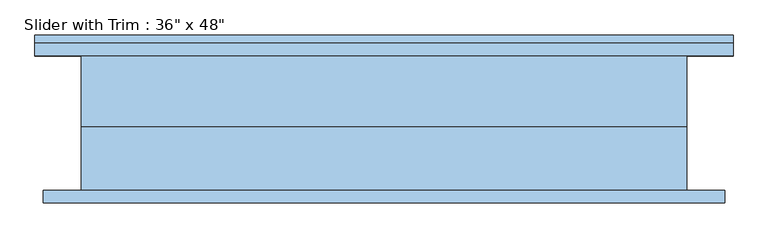
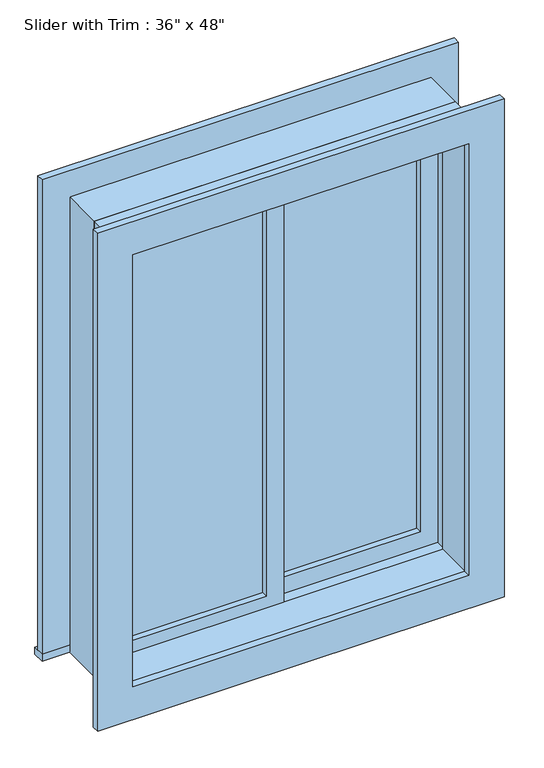
"""IFC4 building model written with IfcOpenShell, lengths in millimetres: window geometry."""

from ifc_helpers import new_model, si_unit, frame, origin, place, context, project, spatial, polyline, outline, extrude, source, transform, mapped, element, save


def window_54100e87(model_context):
    return source(origin(), model_context, "Body", "SweptSolid", [
        extrude(outline(polyline([(-393.7, 22.225), (-22.225, 22.225), (-22.225, 9.525), (-393.7, 9.525), (-393.7, 22.225)])), frame((0.0, 0.0, 977.9), z_axis=(0.0, 0.0, 1.0), x_axis=(1.0, 0.0, 0.0)), (0.0, 0.0, 1.0), 1092.2),
        extrude(outline(polyline([(2114.55, -438.15), (933.45, -438.15), (933.45, 22.225), (2114.55, 22.225), (2114.55, -438.15)]), holes=[polyline([(2070.1, -393.7), (2070.1, -22.225), (977.9, -22.225), (977.9, -393.7), (2070.1, -393.7)])]), frame((0.0, -6.35, 0.0), z_axis=(0.0, 1.0, 0.0), x_axis=(0.0, 0.0, 1.0)), (0.0, 0.0, 1.0), 44.45),
        extrude(outline(polyline([(-527.05, 133.35), (527.05, 133.35), (527.05, 101.6), (-527.05, 101.6), (-527.05, 133.35)])), frame((0.0, 0.0, 914.4), z_axis=(0.0, 0.0, 1.0), x_axis=(1.0, 0.0, 0.0)), (0.0, 0.0, 1.0), 19.05),
        extrude(outline(polyline([(2114.55, -438.15), (2114.55, 438.15), (933.45, 438.15), (933.45, 527.05), (2203.45, 527.05), (2203.45, -527.05), (933.45, -527.05), (933.45, -438.15), (2114.55, -438.15)])), frame((0.0, 101.6, 0.0), z_axis=(0.0, 1.0, 0.0), x_axis=(0.0, 0.0, 1.0)), (0.0, 0.0, 1.0), 19.05),
        extrude(outline(polyline([(2190.75, 514.35), (2190.75, -514.35), (857.25, -514.35), (857.25, 514.35), (2190.75, 514.35)]), holes=[polyline([(2101.85, 425.45), (946.15, 425.45), (946.15, -425.45), (2101.85, -425.45), (2101.85, 425.45)])]), frame((0.0, -120.65, 0.0), z_axis=(0.0, 1.0, 0.0), x_axis=(0.0, 0.0, 1.0)), (0.0, 0.0, 1.0), 19.05),
        extrude(outline(polyline([(393.7, 53.975), (22.225, 53.975), (22.225, 66.675), (393.7, 66.675), (393.7, 53.975)])), frame((0.0, 0.0, 977.9), z_axis=(0.0, 0.0, 1.0), x_axis=(1.0, 0.0, 0.0)), (0.0, 0.0, 1.0), 1092.2),
        extrude(outline(polyline([(2114.55, -22.225), (933.45, -22.225), (933.45, 438.15), (2114.55, 438.15), (2114.55, -22.225)]), holes=[polyline([(2070.1, 22.225), (2070.1, 393.7), (977.9, 393.7), (977.9, 22.225), (2070.1, 22.225)])]), frame((0.0, 38.1, 0.0), z_axis=(0.0, 1.0, 0.0), x_axis=(0.0, 0.0, 1.0)), (0.0, 0.0, 1.0), 44.45),
        extrude(outline(polyline([(2133.6, -457.2), (914.4, -457.2), (914.4, 457.2), (2133.6, 457.2), (2133.6, -457.2)]), holes=[polyline([(2101.85, -425.45), (2101.85, 425.45), (946.15, 425.45), (946.15, -425.45), (2101.85, -425.45)])]), frame((0.0, -101.6, 0.0), z_axis=(0.0, 1.0, 0.0), x_axis=(0.0, 0.0, 1.0)), (0.0, 0.0, 1.0), 95.25),
        extrude(outline(polyline([(2133.6, 457.2), (2133.6, -457.2), (914.4, -457.2), (914.4, 457.2), (2133.6, 457.2)]), holes=[polyline([(2114.55, 438.15), (933.45, 438.15), (933.45, -438.15), (2114.55, -438.15), (2114.55, 438.15)])]), frame((0.0, -6.35, 0.0), z_axis=(0.0, 1.0, 0.0), x_axis=(0.0, 0.0, 1.0)), (0.0, 0.0, 1.0), 107.95),
    ])


if __name__ == "__main__":
    model = new_model("IFC4")
    model_context = context("Model", 3, world=origin())
    ifc_project = project(units=[si_unit("LENGTHUNIT", "METRE", prefix="MILLI")], contexts=[model_context])
    site = spatial("IfcSite", under=ifc_project)
    building = spatial("IfcBuilding", under=site)
    placement = place(None, origin())
    window_shape = window_54100e87(model_context)
    element("IfcWindow", 1, ObjectType="Slider with Trim : 36\" x 48\"", at=placement, inside=building, context=model_context, shape_type="MappedRepresentation", body=[
        mapped(window_shape, transform((0.0, 0.0, 0.0), x_axis=(1.0, 0.0, 0.0), y_axis=(0.0, 1.0, 0.0), z_axis=(0.0, 0.0, 1.0))),
    ])
    save(model, "model.ifc")

# Revit data of these elements
# Type "Slider with Trim : 36\" x 48\""
#   Type Mark = "10"
#   Construction Type Id = "GSP4R"
#   Assembly Code = "B2020100"
#   Analytic Construction = "1/8 in Pilkington single glazing"
#   Visual Light Transmittance = 0.9
#   Solar Heat Gain Coefficient = 0.78
#   Heat Transfer Coefficient (U) = 0.6496 BTU/(h·ft²·°F)
#   Height = 4' - 0"
#   Default Sill Height = 3' - 0"
#   Trim Projection - Ext. = 0' - 0 3/4"
#   Trim Projection - Int. = 0' - 0 3/4"
#   Trim Width - Exterior = 0' - 3 1/2"
#   Trim Width - Interior = 0' - 3 1/2"
#   Width = 3' - 0"
#   Window Inset = 0' - 0 3/4"
#   Define Thermal Properties by = 1
#   Glass Pane Material = Glass
#   Sash Material = Sash
#   Trim Exterior Material = Trim
#   Trim Interior Material = Trim
#   Wall Closure = (empty or 0)
# Element 1 (IfcWindow, "Slider with Trim : 36\" x 48\"")
#   Materials on its faces: "Sash", "Trim", "Glass"
# Materials
#   "Glass": class "Glass", colour RGB 0 128 192, transparency 0.75, Description = "Soda Lime Glass", Cost = 0
#   "Sash": class "Wood", colour RGB 224 178 126, transparency 0
#   "Trim": class "Wood", colour RGB 224 178 126, transparency 0
